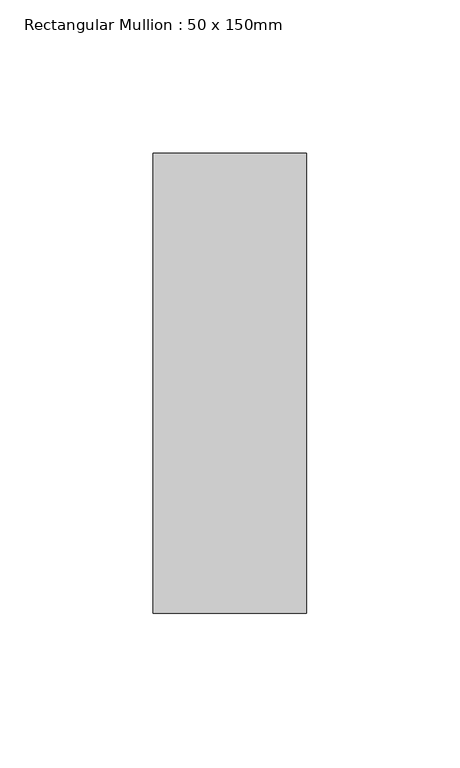
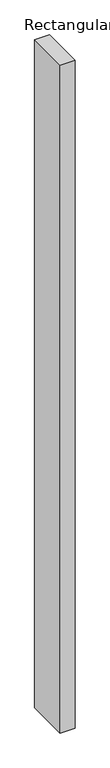
"""IFC4 building model written with IfcOpenShell, lengths in millimetres: member geometry, Rectangular Mullion : 50 x 150mm."""

from ifc_helpers import new_model, si_unit, frame, origin, place, context, project, spatial, polyline, outline, extrude, source, transform, mapped, element, save


def rectangular_mullion_50_x_150mm_6225e4e3(model_context):
    return source(origin(), model_context, "Body", "SweptSolid", [
        extrude(outline(polyline([(25.0, 75.0), (25.0, -75.0), (-25.0, -75.0), (-25.0, 75.0), (25.0, 75.0)])), frame((0.0, 0.0, -2400.0), z_axis=(0.0, 0.0, 1.0), x_axis=(1.0, 0.0, 0.0)), (0.0, 0.0, 1.0), 2400.0),
    ])


if __name__ == "__main__":
    model = new_model("IFC4")
    model_context = context("Model", 3, world=origin())
    ifc_project = project(units=[si_unit("LENGTHUNIT", "METRE", prefix="MILLI")], contexts=[model_context])
    site = spatial("IfcSite", under=ifc_project)
    building = spatial("IfcBuilding", under=site)
    placement = place(None, origin())
    rectangular_mullion_50_x_150mm_shape = rectangular_mullion_50_x_150mm_6225e4e3(model_context)
    element("IfcMember", 1, ObjectType="Rectangular Mullion : 50 x 150mm", at=placement, inside=building, context=model_context, shape_type="MappedRepresentation", body=[
        mapped(rectangular_mullion_50_x_150mm_shape, transform((0.0, 0.0, 0.0), x_axis=(1.0, 0.0, 0.0), y_axis=(0.0, 1.0, 0.0), z_axis=(0.0, 0.0, 1.0))),
    ])
    save(model, "model.ifc")

# Revit data of these elements
# Type "Rectangular Mullion : 50 x 150mm"
#   built-in parameter 1007304 = 0.492126 (stored number, unit not read)
#   built-in parameter 1007301 = 0.082021 (stored number, unit not read)
#   built-in parameter 1007300 = 0.082021 (stored number, unit not read)
# Element 1 (IfcMember, "Rectangular Mullion : 50 x 150mm")
#   Materials on its faces: "Aluminium"
# Materials
#   "Aluminium": class "Metal", colour RGB 247 247 247, transparency 0, Description = "Aluminium 6061", Cost = 0
